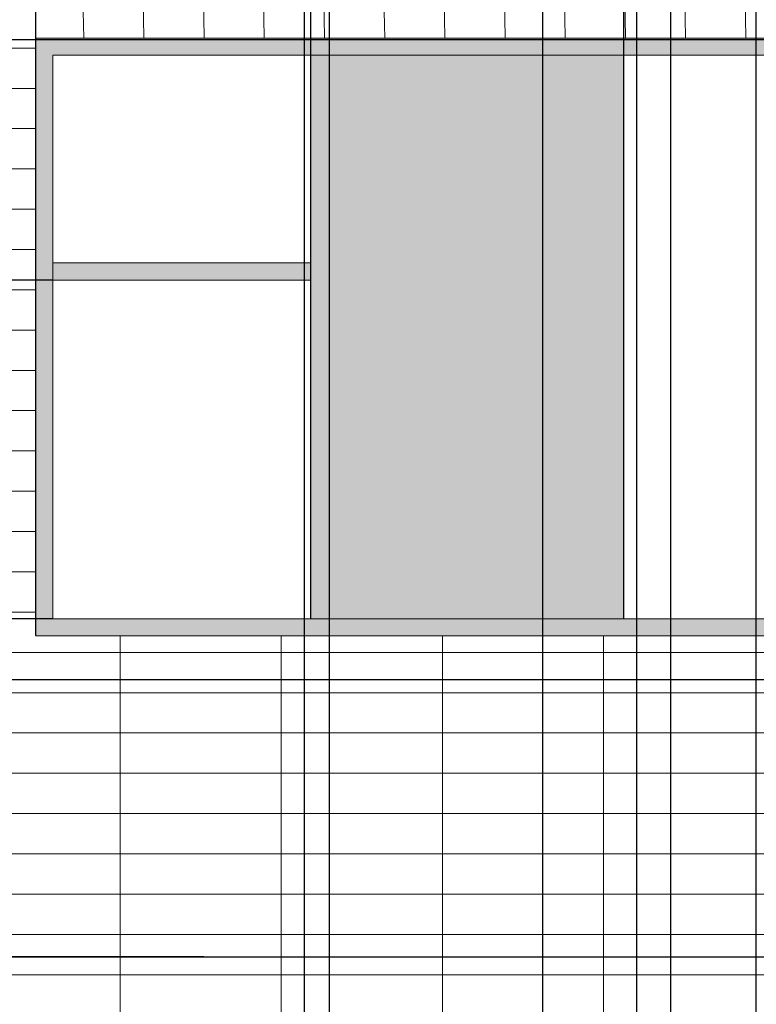
# Model space of a CAD drawing. Units: inches. Extents: x 241 to 943, y 109 to 1396.
# Tile 29 of 34: x 532 to 618, y 1065 to 1180. Entities that reach past the tile are written whole.
import ezdxf

# ---------------------------------------------------------------- set-up
doc = ezdxf.new("R2010")
doc.units = ezdxf.units.IN
doc.header["$MEASUREMENT"] = 0
for name, color, linetype, lineweight in [('A-ANNO-DIMS', 2, 'Continuous', 18), ('A-ELEV', 7, 'Continuous', 25), ('A-ELEV-SHAD', 9, 'Continuous', 13), ('A-GLAZ', 4, 'Continuous', 18), ('A-GLAZ-PATT', 18, 'Continuous', 13), ('A-WALL-PATT', 8, 'Continuous', 13)]:
    doc.layers.add(name, color=color, linetype=linetype, lineweight=lineweight)
doc.styles.get("Standard").update_dxf_attribs({"font": 'arial.ttf'})
doc.dimstyles.get("Standard").update_dxf_attribs({"dimtxt": 1.4375, "dimasz": 0.18, "dimexe": 0.18, "dimexo": 0.0625, "dimgap": 0.09, "dimtad": 0, "dimtih": 1, "dimtoh": 1, "dimdec": 4, "dimzin": 0, "dimdsep": 46, "dimlunit": 4, "dimtxsty": 'Standard', "dimcen": 0.09, "dimadec": 0, "dimazin": 0, "dimtfac": 1, "dimtdec": 4, "dimtofl": 0, "dimtmove": 0, "dimatfit": 3, "dimfxl": 1, "dimtolj": 1, "dimtzin": 0, "dimarcsym": 0})

# ---------------------------------------------------------------- blocks, each defined once
blk = doc.blocks.new('*D12')
at = {"layer": 'A-ANNO-DIMS', "color": 0, "lineweight": -2, "transparency": 16777216}
for p, q in [((530.23, 384.24), (530.23, 1395.05)), ((530.41, 1394.87), (587.56, 1394.87)), ((650.73, 1394.87), (593.58, 1394.87)), ((650.91, 384.24), (650.91, 1395.05))]:
    blk.add_line(p, q, dxfattribs=at)
at = {"layer": 'A-ANNO-DIMS', "color": 0, "transparency": 16777216}
for points in [[(530.41, 1394.9), (530.41, 1394.84), (530.23, 1394.87)], [(650.73, 1394.9), (650.73, 1394.84), (650.91, 1394.87)]]:
    blk.add_solid(points, dxfattribs=at)
at = {"layer": 'Defpoints', "color": 0, "transparency": 16777216}
for p in [(650.91, 1394.87), (530.23, 384.18), (650.91, 384.18)]:
    blk.add_point(p, dxfattribs=at)
at = {"layer": 'A-ANNO-DIMS', "color": 0, "transparency": 16777216, "insert": (590.57, 1394.87), "char_height": 1.438, "attachment_point": 5}
blk.add_mtext('\\A1;120.68', dxfattribs=at)
blk = doc.blocks.new('*D49')
at = {"layer": 'A-ANNO-DIMS', "color": 0, "lineweight": -2, "transparency": 16777216}
for p, q in [((766.24, 1177.54), (244.31, 1177.54)), ((244.49, 1177.36), (244.49, 1141.12)), ((244.49, 1103.23), (244.49, 1139.47)), ((766.24, 1103.05), (244.31, 1103.05))]:
    blk.add_line(p, q, dxfattribs=at)
at = {"layer": 'A-ANNO-DIMS', "color": 0, "transparency": 16777216}
for points in [[(244.46, 1177.36), (244.52, 1177.36), (244.49, 1177.54)], [(244.46, 1103.23), (244.52, 1103.23), (244.49, 1103.05)]]:
    blk.add_solid(points, dxfattribs=at)
at = {"layer": 'Defpoints', "color": 0, "transparency": 16777216}
for p in [(244.49, 1177.54), (766.3, 1177.54), (766.3, 1103.05)]:
    blk.add_point(p, dxfattribs=at)
at = {"layer": 'A-ANNO-DIMS', "color": 0, "transparency": 16777216, "insert": (244.49, 1140.29), "char_height": 1.438, "attachment_point": 5}
blk.add_mtext('\\A1;74.49', dxfattribs=at)
blk = doc.blocks.new('*D57')
at = {"layer": 'A-ANNO-DIMS', "color": 0, "lineweight": -2, "transparency": 16777216}
for p, q in [((508.31, 1070.92), (508.31, 1395.05)), ((508.49, 1394.87), (518.04, 1394.87)), ((533.77, 1394.87), (524.21, 1394.87)), ((533.95, 1108.23), (533.95, 1395.05))]:
    blk.add_line(p, q, dxfattribs=at)
at = {"layer": 'A-ANNO-DIMS', "color": 0, "transparency": 16777216}
for points in [[(508.49, 1394.9), (508.49, 1394.84), (508.31, 1394.87)], [(533.77, 1394.9), (533.77, 1394.84), (533.95, 1394.87)]]:
    blk.add_solid(points, dxfattribs=at)
at = {"layer": 'Defpoints', "color": 0, "transparency": 16777216}
for p in [(533.95, 1394.87), (533.95, 1108.17), (508.31, 1070.85)]:
    blk.add_point(p, dxfattribs=at)
at = {"layer": 'A-ANNO-DIMS', "color": 0, "transparency": 16777216, "insert": (521.13, 1394.87), "char_height": 1.438, "attachment_point": 5}
blk.add_mtext('\\A1;25.646', dxfattribs=at)
blk = doc.blocks.new('*D62')
at = {"layer": 'A-ANNO-DIMS', "color": 0, "lineweight": -2, "transparency": 16777216}
for p, q in [((424.11, 568.89), (424.11, 1395.05)), ((424.29, 1394.87), (492.35, 1394.87)), ((565.02, 1394.87), (496.96, 1394.87)), ((565.2, 568.89), (565.2, 1395.05))]:
    blk.add_line(p, q, dxfattribs=at)
at = {"layer": 'A-ANNO-DIMS', "color": 0, "transparency": 16777216}
for points in [[(424.29, 1394.9), (424.29, 1394.84), (424.11, 1394.87)], [(565.02, 1394.9), (565.02, 1394.84), (565.2, 1394.87)]]:
    blk.add_solid(points, dxfattribs=at)
at = {"layer": 'Defpoints', "color": 0, "transparency": 16777216}
for p in [(565.2, 1394.87), (424.11, 568.83), (565.2, 568.83)]:
    blk.add_point(p, dxfattribs=at)
at = {"layer": 'A-ANNO-DIMS', "color": 0, "transparency": 16777216, "insert": (494.66, 1394.87), "char_height": 1.438, "attachment_point": 5}
blk.add_mtext('\\A1;141.1', dxfattribs=at)
blk = doc.blocks.new('*D65')
at = {"layer": 'A-ANNO-DIMS', "color": 0, "lineweight": -2, "transparency": 16777216}
for p, q in [((424.11, 700.85), (424.11, 1395.05)), ((424.29, 1394.87), (505.52, 1394.87)), ((592.77, 1394.87), (511.54, 1394.87)), ((592.95, 700.85), (592.95, 1395.05))]:
    blk.add_line(p, q, dxfattribs=at)
at = {"layer": 'A-ANNO-DIMS', "color": 0, "transparency": 16777216}
for points in [[(424.29, 1394.9), (424.29, 1394.84), (424.11, 1394.87)], [(592.77, 1394.9), (592.77, 1394.84), (592.95, 1394.87)]]:
    blk.add_solid(points, dxfattribs=at)
at = {"layer": 'Defpoints', "color": 0, "transparency": 16777216}
for p in [(592.95, 1394.87), (424.11, 700.79), (592.95, 700.79)]:
    blk.add_point(p, dxfattribs=at)
at = {"layer": 'A-ANNO-DIMS', "color": 0, "transparency": 16777216, "insert": (508.53, 1394.87), "char_height": 1.438, "attachment_point": 5}
blk.add_mtext('\\A1;168.85', dxfattribs=at)
blk = doc.blocks.new('*D66')
at = {"layer": 'A-ANNO-DIMS', "color": 0, "lineweight": -2, "transparency": 16777216}
for p, q in [((617.76, 702.85), (617.76, 1395.05)), ((617.94, 1394.87), (680.69, 1394.87)), ((749.45, 1394.87), (686.7, 1394.87)), ((749.63, 702.85), (749.63, 1395.05))]:
    blk.add_line(p, q, dxfattribs=at)
at = {"layer": 'A-ANNO-DIMS', "color": 0, "transparency": 16777216}
for points in [[(617.94, 1394.9), (617.94, 1394.84), (617.76, 1394.87)], [(749.45, 1394.9), (749.45, 1394.84), (749.63, 1394.87)]]:
    blk.add_solid(points, dxfattribs=at)
at = {"layer": 'Defpoints', "color": 0, "transparency": 16777216}
for p in [(749.63, 1394.87), (617.76, 702.79), (749.63, 702.79)]:
    blk.add_point(p, dxfattribs=at)
at = {"layer": 'A-ANNO-DIMS', "color": 0, "transparency": 16777216, "insert": (683.7, 1394.87), "char_height": 1.438, "attachment_point": 5}
blk.add_mtext('\\A1;131.87', dxfattribs=at)
blk = doc.blocks.new('*D67')
at = {"layer": 'A-ANNO-DIMS', "color": 0, "lineweight": -2, "transparency": 16777216}
for p, q in [((389.04, 773.55), (389.04, 1395.05)), ((389.22, 1394.87), (495.34, 1394.87)), ((607.64, 1394.87), (501.52, 1394.87)), ((607.82, 773.55), (607.82, 1395.05))]:
    blk.add_line(p, q, dxfattribs=at)
at = {"layer": 'A-ANNO-DIMS', "color": 0, "transparency": 16777216}
for points in [[(389.22, 1394.9), (389.22, 1394.84), (389.04, 1394.87)], [(607.64, 1394.9), (607.64, 1394.84), (607.82, 1394.87)]]:
    blk.add_solid(points, dxfattribs=at)
at = {"layer": 'Defpoints', "color": 0, "transparency": 16777216}
for p in [(607.82, 1394.87), (389.04, 773.49), (607.82, 773.49)]:
    blk.add_point(p, dxfattribs=at)
at = {"layer": 'A-ANNO-DIMS', "color": 0, "transparency": 16777216, "insert": (498.43, 1394.87), "char_height": 1.438, "attachment_point": 5}
blk.add_mtext('\\A1;218.77', dxfattribs=at)
blk = doc.blocks.new('*D68')
at = {"layer": 'A-ANNO-DIMS', "color": 0, "lineweight": -2, "transparency": 16777216}
for p, q in [((617.76, 841.6), (617.76, 1395.05)), ((617.94, 1394.87), (702.22, 1394.87)), ((792.51, 1394.87), (708.23, 1394.87)), ((792.69, 841.6), (792.69, 1395.05))]:
    blk.add_line(p, q, dxfattribs=at)
at = {"layer": 'A-ANNO-DIMS', "color": 0, "transparency": 16777216}
for points in [[(617.94, 1394.9), (617.94, 1394.84), (617.76, 1394.87)], [(792.51, 1394.9), (792.51, 1394.84), (792.69, 1394.87)]]:
    blk.add_solid(points, dxfattribs=at)
at = {"layer": 'Defpoints', "color": 0, "transparency": 16777216}
for p in [(792.69, 1394.87), (617.76, 841.54), (792.69, 841.54)]:
    blk.add_point(p, dxfattribs=at)
at = {"layer": 'A-ANNO-DIMS', "color": 0, "transparency": 16777216, "insert": (705.23, 1394.87), "char_height": 1.438, "attachment_point": 5}
blk.add_mtext('\\A1;174.93', dxfattribs=at)
blk = doc.blocks.new('*D69')
at = {"layer": 'A-ANNO-DIMS', "color": 0, "lineweight": -2, "transparency": 16777216}
for p, q in [((389.04, 941.55), (389.04, 1395.05)), ((389.22, 1394.87), (476.28, 1394.87)), ((567.95, 1394.87), (480.9, 1394.87)), ((568.13, 941.55), (568.13, 1395.05))]:
    blk.add_line(p, q, dxfattribs=at)
at = {"layer": 'A-ANNO-DIMS', "color": 0, "transparency": 16777216}
for points in [[(389.22, 1394.9), (389.22, 1394.84), (389.04, 1394.87)], [(567.95, 1394.9), (567.95, 1394.84), (568.13, 1394.87)]]:
    blk.add_solid(points, dxfattribs=at)
at = {"layer": 'Defpoints', "color": 0, "transparency": 16777216}
for p in [(568.13, 1394.87), (389.04, 941.49), (568.13, 941.49)]:
    blk.add_point(p, dxfattribs=at)
at = {"layer": 'A-ANNO-DIMS', "color": 0, "transparency": 16777216, "insert": (478.59, 1394.87), "char_height": 1.438, "attachment_point": 5}
blk.add_mtext('\\A1;179.1', dxfattribs=at)
blk = doc.blocks.new('*D70')
at = {"layer": 'A-ANNO-DIMS', "color": 0, "lineweight": -2, "transparency": 16777216}
for p, q in [((603.87, 1009.6), (603.87, 1395.05)), ((604.05, 1394.87), (674.69, 1394.87)), ((751.33, 1394.87), (680.69, 1394.87)), ((751.51, 1009.6), (751.51, 1395.05))]:
    blk.add_line(p, q, dxfattribs=at)
at = {"layer": 'A-ANNO-DIMS', "color": 0, "transparency": 16777216}
for points in [[(604.05, 1394.9), (604.05, 1394.84), (603.87, 1394.87)], [(751.33, 1394.9), (751.33, 1394.84), (751.51, 1394.87)]]:
    blk.add_solid(points, dxfattribs=at)
at = {"layer": 'Defpoints', "color": 0, "transparency": 16777216}
for p in [(751.51, 1394.87), (603.87, 1009.54), (751.51, 1009.54)]:
    blk.add_point(p, dxfattribs=at)
at = {"layer": 'A-ANNO-DIMS', "color": 0, "transparency": 16777216, "insert": (677.69, 1394.87), "char_height": 1.438, "attachment_point": 5}
blk.add_mtext('\\A1;147.64', dxfattribs=at)
blk = doc.blocks.new('*D82')
at = {"layer": 'A-ANNO-DIMS', "color": 0, "lineweight": -2, "transparency": 16777216}
for p, q in [((565.2, 568.89), (565.2, 1395.05)), ((565.38, 1394.87), (605.89, 1394.87)), ((651.42, 1394.87), (610.91, 1394.87)), ((651.6, 568.89), (651.6, 1395.05))]:
    blk.add_line(p, q, dxfattribs=at)
at = {"layer": 'A-ANNO-DIMS', "color": 0, "transparency": 16777216}
for points in [[(565.38, 1394.9), (565.38, 1394.84), (565.2, 1394.87)], [(651.42, 1394.9), (651.42, 1394.84), (651.6, 1394.87)]]:
    blk.add_solid(points, dxfattribs=at)
at = {"layer": 'Defpoints', "color": 0, "transparency": 16777216}
for p in [(651.6, 1394.87), (565.2, 568.83), (651.6, 568.83)]:
    blk.add_point(p, dxfattribs=at)
at = {"layer": 'A-ANNO-DIMS', "color": 0, "transparency": 16777216, "insert": (608.4, 1394.87), "char_height": 1.438, "attachment_point": 5}
blk.add_mtext('\\A1;86.40', dxfattribs=at)
blk = doc.blocks.new('*D83')
at = {"layer": 'A-ANNO-DIMS', "color": 0, "lineweight": -2, "transparency": 16777216}
for p, q in [((592.95, 700.85), (592.95, 1395.05)), ((593.13, 1394.87), (602.27, 1394.87)), ((617.58, 1394.87), (608.45, 1394.87)), ((617.76, 702.85), (617.76, 1395.05))]:
    blk.add_line(p, q, dxfattribs=at)
at = {"layer": 'A-ANNO-DIMS', "color": 0, "transparency": 16777216}
for points in [[(593.13, 1394.9), (593.13, 1394.84), (592.95, 1394.87)], [(617.58, 1394.9), (617.58, 1394.84), (617.76, 1394.87)]]:
    blk.add_solid(points, dxfattribs=at)
at = {"layer": 'Defpoints', "color": 0, "transparency": 16777216}
for p in [(617.76, 1394.87), (617.76, 702.79), (592.95, 700.79)]:
    blk.add_point(p, dxfattribs=at)
at = {"layer": 'A-ANNO-DIMS', "color": 0, "transparency": 16777216, "insert": (605.36, 1394.87), "char_height": 1.438, "attachment_point": 5}
blk.add_mtext('\\A1;24.805', dxfattribs=at)
blk = doc.blocks.new('*D89')
at = {"layer": 'A-ANNO-DIMS', "color": 0, "lineweight": -2, "transparency": 16777216}
for p, q in [((377.04, 841.6), (377.04, 1395.05)), ((377.22, 1394.87), (494.32, 1394.87)), ((617.58, 1394.87), (500.48, 1394.87)), ((617.76, 841.6), (617.76, 1395.05))]:
    blk.add_line(p, q, dxfattribs=at)
at = {"layer": 'A-ANNO-DIMS', "color": 0, "transparency": 16777216}
for points in [[(377.22, 1394.9), (377.22, 1394.84), (377.04, 1394.87)], [(617.58, 1394.9), (617.58, 1394.84), (617.76, 1394.87)]]:
    blk.add_solid(points, dxfattribs=at)
at = {"layer": 'Defpoints', "color": 0, "transparency": 16777216}
for p in [(617.76, 1394.87), (377.04, 841.54), (617.76, 841.54)]:
    blk.add_point(p, dxfattribs=at)
at = {"layer": 'A-ANNO-DIMS', "color": 0, "transparency": 16777216, "insert": (497.4, 1394.87), "char_height": 1.438, "attachment_point": 5}
blk.add_mtext('\\A1;240.72', dxfattribs=at)
blk = doc.blocks.new('*D90')
at = {"layer": 'A-ANNO-DIMS', "color": 0, "lineweight": -2, "transparency": 16777216}
for p, q in [((568.13, 941.55), (568.13, 1395.05)), ((568.31, 1394.87), (582.92, 1394.87)), ((603.69, 1394.87), (589.08, 1394.87)), ((603.87, 902.92), (603.87, 1395.05))]:
    blk.add_line(p, q, dxfattribs=at)
at = {"layer": 'A-ANNO-DIMS', "color": 0, "transparency": 16777216}
for points in [[(568.31, 1394.9), (568.31, 1394.84), (568.13, 1394.87)], [(603.69, 1394.9), (603.69, 1394.84), (603.87, 1394.87)]]:
    blk.add_solid(points, dxfattribs=at)
at = {"layer": 'Defpoints', "color": 0, "transparency": 16777216}
for p in [(603.87, 1394.87), (568.13, 941.49), (603.87, 902.85)]:
    blk.add_point(p, dxfattribs=at)
at = {"layer": 'A-ANNO-DIMS', "color": 0, "transparency": 16777216, "insert": (586, 1394.87), "char_height": 1.438, "attachment_point": 5}
blk.add_mtext('\\A1;35.735', dxfattribs=at)
blk = doc.blocks.new('*D95')
at = {"layer": 'A-ANNO-DIMS', "color": 0, "lineweight": -2, "transparency": 16777216}
for p, q in [((724.88, 1108.17), (940.6, 1108.17)), ((940.42, 1107.99), (940.42, 1090.34)), ((940.42, 1071.03), (940.42, 1088.69)), ((508.37, 1070.85), (940.6, 1070.85))]:
    blk.add_line(p, q, dxfattribs=at)
at = {"layer": 'A-ANNO-DIMS', "color": 0, "transparency": 16777216}
for points in [[(940.39, 1107.99), (940.45, 1107.99), (940.42, 1108.17)], [(940.39, 1071.03), (940.45, 1071.03), (940.42, 1070.85)]]:
    blk.add_solid(points, dxfattribs=at)
at = {"layer": 'Defpoints', "color": 0, "transparency": 16777216}
for p in [(724.82, 1108.17), (940.42, 1108.17), (508.31, 1070.85)]:
    blk.add_point(p, dxfattribs=at)
at = {"layer": 'A-ANNO-DIMS', "color": 0, "transparency": 16777216, "insert": (940.42, 1089.51), "char_height": 1.438, "attachment_point": 5}
blk.add_mtext('\\A1;37.315', dxfattribs=at)
blk = doc.blocks.new('*D99')
at = {"layer": 'A-ANNO-DIMS', "color": 0, "lineweight": -2, "transparency": 16777216}
for p, q in [((417.09, 181.71), (417.09, 1395.05)), ((417.27, 1394.87), (539.16, 1394.87)), ((667.21, 1394.87), (545.33, 1394.87)), ((667.39, 214.58), (667.39, 1395.05))]:
    blk.add_line(p, q, dxfattribs=at)
at = {"layer": 'A-ANNO-DIMS', "color": 0, "transparency": 16777216}
for points in [[(417.27, 1394.9), (417.27, 1394.84), (417.09, 1394.87)], [(667.21, 1394.9), (667.21, 1394.84), (667.39, 1394.87)]]:
    blk.add_solid(points, dxfattribs=at)
at = {"layer": 'Defpoints', "color": 0, "transparency": 16777216}
for p in [(667.39, 1394.87), (667.39, 214.52), (417.09, 181.65)]:
    blk.add_point(p, dxfattribs=at)
at = {"layer": 'A-ANNO-DIMS', "color": 0, "transparency": 16777216, "insert": (542.24, 1394.87), "char_height": 1.438, "attachment_point": 5}
blk.add_mtext('\\A1;250.30', dxfattribs=at)
blk = doc.blocks.new('*D104')
at = {"layer": 'A-ANNO-DIMS', "color": 0, "lineweight": -2, "transparency": 16777216}
for p, q in [((533.95, 1108.23), (533.95, 1395.05)), ((534.13, 1394.87), (546.87, 1394.87)), ((565.77, 1394.87), (553.03, 1394.87)), ((565.95, 1110.23), (565.95, 1395.05))]:
    blk.add_line(p, q, dxfattribs=at)
at = {"layer": 'A-ANNO-DIMS', "color": 0, "transparency": 16777216}
for points in [[(534.13, 1394.9), (534.13, 1394.84), (533.95, 1394.87)], [(565.77, 1394.9), (565.77, 1394.84), (565.95, 1394.87)]]:
    blk.add_solid(points, dxfattribs=at)
at = {"layer": 'Defpoints', "color": 0, "transparency": 16777216}
for p in [(565.95, 1394.87), (565.95, 1110.17), (533.95, 1108.17)]:
    blk.add_point(p, dxfattribs=at)
at = {"layer": 'A-ANNO-DIMS', "color": 0, "transparency": 16777216, "insert": (549.95, 1394.87), "char_height": 1.438, "attachment_point": 5}
blk.add_mtext('\\A1;31.995', dxfattribs=at)
blk = doc.blocks.new('*D105')
at = {"layer": 'A-ANNO-DIMS', "color": 0, "lineweight": -2, "transparency": 16777216}
for p, q in [((565.95, 1110.23), (565.95, 1395.05)), ((566.13, 1394.87), (581.08, 1394.87)), ((602.18, 1394.87), (587.23, 1394.87)), ((602.36, 1110.23), (602.36, 1395.05))]:
    blk.add_line(p, q, dxfattribs=at)
at = {"layer": 'A-ANNO-DIMS', "color": 0, "transparency": 16777216}
for points in [[(566.13, 1394.9), (566.13, 1394.84), (565.95, 1394.87)], [(602.18, 1394.9), (602.18, 1394.84), (602.36, 1394.87)]]:
    blk.add_solid(points, dxfattribs=at)
at = {"layer": 'Defpoints', "color": 0, "transparency": 16777216}
for p in [(602.36, 1394.87), (565.95, 1110.17), (602.36, 1110.17)]:
    blk.add_point(p, dxfattribs=at)
at = {"layer": 'A-ANNO-DIMS', "color": 0, "transparency": 16777216, "insert": (584.15, 1394.87), "char_height": 1.438, "attachment_point": 5}
blk.add_mtext('\\A1;36.415', dxfattribs=at)
blk = doc.blocks.new('*D106')
at = {"layer": 'A-ANNO-DIMS', "color": 0, "lineweight": -2, "transparency": 16777216}
for p, q in [((602.36, 1110.23), (602.36, 1395.05)), ((602.54, 1394.87), (608.99, 1394.87)), ((620.34, 1394.87), (613.89, 1394.87)), ((620.52, 1110.23), (620.52, 1395.05))]:
    blk.add_line(p, q, dxfattribs=at)
at = {"layer": 'A-ANNO-DIMS', "color": 0, "transparency": 16777216}
for points in [[(602.54, 1394.9), (602.54, 1394.84), (602.36, 1394.87)], [(620.34, 1394.9), (620.34, 1394.84), (620.52, 1394.87)]]:
    blk.add_solid(points, dxfattribs=at)
at = {"layer": 'Defpoints', "color": 0, "transparency": 16777216}
for p in [(620.52, 1394.87), (602.36, 1110.17), (620.52, 1110.17)]:
    blk.add_point(p, dxfattribs=at)
at = {"layer": 'A-ANNO-DIMS', "color": 0, "transparency": 16777216, "insert": (611.44, 1394.87), "char_height": 1.438, "attachment_point": 5}
blk.add_mtext('\\A1;18.16', dxfattribs=at)
blk = doc.blocks.new('*D110')
at = {"layer": 'A-ANNO-DIMS', "color": 0, "lineweight": -2, "transparency": 16777216}
for p, q in [((535.89, 1149.58), (244.31, 1149.58)), ((244.49, 1149.4), (244.49, 1130.7)), ((244.49, 1110.35), (244.49, 1129.05)), ((535.89, 1110.17), (244.31, 1110.17))]:
    blk.add_line(p, q, dxfattribs=at)
at = {"layer": 'A-ANNO-DIMS', "color": 0, "transparency": 16777216}
for points in [[(244.46, 1149.4), (244.52, 1149.4), (244.49, 1149.58)], [(244.46, 1110.35), (244.52, 1110.35), (244.49, 1110.17)]]:
    blk.add_solid(points, dxfattribs=at)
at = {"layer": 'Defpoints', "color": 0, "transparency": 16777216}
for p in [(244.49, 1149.58), (535.95, 1149.58), (535.95, 1110.17)]:
    blk.add_point(p, dxfattribs=at)
at = {"layer": 'A-ANNO-DIMS', "color": 0, "transparency": 16777216, "insert": (244.49, 1129.87), "char_height": 1.438, "attachment_point": 5}
blk.add_mtext('\\A1;39.41', dxfattribs=at)
blk = doc.blocks.new('*D113')
at = {"layer": 'A-ANNO-DIMS', "color": 0, "lineweight": -2, "transparency": 16777216}
for p, q in [((603.87, 902.92), (603.87, 1395.05)), ((604.05, 1394.87), (618.91, 1394.87)), ((639.93, 1394.87), (625.07, 1394.87)), ((640.11, 902.92), (640.11, 1395.05))]:
    blk.add_line(p, q, dxfattribs=at)
at = {"layer": 'A-ANNO-DIMS', "color": 0, "transparency": 16777216}
for points in [[(604.05, 1394.9), (604.05, 1394.84), (603.87, 1394.87)], [(639.93, 1394.9), (639.93, 1394.84), (640.11, 1394.87)]]:
    blk.add_solid(points, dxfattribs=at)
at = {"layer": 'Defpoints', "color": 0, "transparency": 16777216}
for p in [(640.11, 1394.87), (603.87, 902.85), (640.11, 902.85)]:
    blk.add_point(p, dxfattribs=at)
at = {"layer": 'A-ANNO-DIMS', "color": 0, "transparency": 16777216, "insert": (621.99, 1394.87), "char_height": 1.438, "attachment_point": 5}
blk.add_mtext('\\A1;36.245', dxfattribs=at)

msp = doc.modelspace()

# ---------------------------------------------------------------- hatches: boundary and pattern name
at = {"layer": 'A-ELEV-SHAD'}
h = msp.add_hatch(color=256, dxfattribs=at)
h.dxf.hatch_style = 1
h.paths.add_polyline_path([(537.4269, 698.7912), (534.1778, 698.7912), (534.1778, 659.3434), (537.4269, 659.3434)])
h.paths.add_polyline_path([(508.0803, 698.7912), (450.9259, 698.7912), (450.9259, 659.3434), (452.9259, 659.3434), (452.9259, 696.7912), (506.0803, 696.7912), (506.0803, 659.3434), (508.0803, 659.3434)])
h.paths.add_polyline_path([(481.5031, 696.7912), (479.5031, 696.7912), (479.5031, 659.3434), (481.5031, 659.3434)], flags=17)
h.paths.add_polyline_path([(481.5031, 657.3434), (479.5031, 657.3434), (479.5031, 653.3371), (481.5031, 653.3371)], flags=17)
h.paths.add_polyline_path([(508.0803, 657.3434), (506.0803, 657.3434), (506.0803, 653.3371), (452.9259, 653.3371), (452.9259, 657.3434), (450.9259, 657.3434), (450.9259, 651.3371), (508.0803, 651.3371)])
h.paths.add_polyline_path([(428.1173, 839.5382), (426.1173, 839.5382), (426.1173, 786.9154), (428.1173, 786.9154)], flags=17)
h.paths.add_polyline_path([(470.8692, 839.5382), (468.8692, 839.5382), (468.8692, 786.9154), (470.8692, 786.9154)], flags=17)
h.paths.add_polyline_path([(508.3064, 841.5382), (396.3125, 841.5382), (396.3125, 782.5808), (398.3125, 782.5808), (398.3125, 839.5382), (506.3064, 839.5382), (506.3064, 782.5808), (508.3064, 782.5808)])
h.paths.add_polyline_path([(398.3125, 780.5808), (396.3125, 780.5808), (396.3125, 773.4916), (398.3125, 773.4916)])
h.paths.add_polyline_path([(508.3064, 780.5808), (506.3064, 780.5808), (506.3064, 773.4916), (508.3064, 773.4916)])
h.paths.add_polyline_path([(715.6236, 841.5382), (678.2674, 841.5382), (678.2674, 734.8538), (715.6236, 734.8538)])
h.paths.add_polyline_path([(680.2674, 839.5382), (682.4526, 839.5382), (713.6236, 839.5382), (713.6236, 736.9235), (690.2047, 736.9235), (680.2674, 736.9235)], flags=16)
h.paths.add_polyline_path([(792.691, 841.5382), (747.7579, 841.5382), (747.7579, 734.8538), (754.5373, 734.8538), (754.5373, 736.9235), (754.5373, 839.5382), (756.7224, 839.5382), (787.8934, 839.5382), (787.8934, 765.9585), (792.691, 765.9585)])
h.paths.add_polyline_path([(659.2925, 1009.5382), (657.2925, 1009.5382), (657.2925, 902.8538), (659.2925, 902.8538)])
h.paths.add_polyline_path([(751.5078, 976.6275), (712.5839, 976.6275), (712.5839, 974.6275), (751.5078, 974.6275)])
h.paths.add_polyline_path([(470.8692, 1007.5382), (468.8692, 1007.5382), (468.8692, 954.9154), (470.8692, 954.9154)], flags=17)
h.paths.add_polyline_path([(508.3064, 1009.5382), (396.3125, 1009.5382), (396.3125, 950.5808), (398.3125, 950.5808), (398.3125, 1007.5382), (506.3064, 1007.5382), (506.3064, 950.5808), (508.3064, 950.5808)])
h.paths.add_polyline_path([(428.1173, 1007.5382), (426.1173, 1007.5382), (426.1173, 954.9154), (428.1173, 954.9154)], flags=17)
h.paths.add_polyline_path([(398.3125, 948.5808), (396.3125, 948.5808), (396.3125, 941.4916), (398.3125, 941.4916)])
h.paths.add_polyline_path([(508.3064, 948.5808), (506.3064, 948.5808), (506.3064, 941.4916), (508.3064, 941.4916)])
h.paths.add_polyline_path([(428.1173, 1175.5382), (426.1173, 1175.5382), (426.1173, 1122.9154), (428.1173, 1122.9154)], flags=17)
h.paths.add_polyline_path([(508.3064, 1177.5382), (396.3125, 1177.5382), (396.3125, 1118.5808), (398.3125, 1118.5808), (398.3125, 1175.5382), (506.3064, 1175.5382), (506.3064, 1118.5808), (506.8039, 1118.5808, -1), (506.8039, 1116.5808), (506.3064, 1116.5808), (506.3064, 1109.4916), (508.3064, 1109.4916)])
h.paths.add_polyline_path([(470.8692, 1175.5382), (468.8692, 1175.5382), (468.8692, 1122.9154), (470.8692, 1122.9154)], flags=17)
h.paths.add_polyline_path([(398.3125, 1116.5808), (396.3125, 1116.5808), (396.3125, 1109.4916), (398.3125, 1109.4916)], flags=17)
h.paths.add_polyline_path([(724.819, 1177.7336), (533.952, 1177.7336), (533.952, 1108.1686), (724.819, 1108.1686)])
h.paths.add_polyline_path([(535.952, 1175.7336), (722.819, 1175.7336), (722.819, 1110.1686), (535.952, 1110.1686)], flags=0)
h.paths.add_polyline_path([(622.521, 1136.0739), (643.4534, 1136.0739), (643.4534, 1134.0739), (622.521, 1134.0739)], flags=0)
h.paths.add_polyline_path([(722.819, 1175.7336), (535.952, 1175.7336), (535.952, 1110.1686), (722.819, 1110.1686)], flags=16)
h.paths.add_polyline_path([(565.947, 1151.5772), (535.952, 1151.5772), (535.952, 1149.5772), (565.947, 1149.5772)], flags=0)
h = msp.add_hatch(color=256, dxfattribs=at)
h.dxf.hatch_style = 1
h.paths.add_polyline_path([(804.5268, 1142.2929), (768.3038, 1142.2929), (768.3038, 1140.2929), (804.5268, 1140.2929)], flags=0)
h.paths.add_polyline_path([(806.5268, 1177.5382), (766.3038, 1177.5382), (766.3038, 1103.0477), (806.5268, 1103.0477)])
h.paths.add_polyline_path([(768.3038, 1175.5382), (804.5268, 1175.5382), (804.5268, 1105.0477), (768.3038, 1105.0477)], flags=16)
h.paths.add_polyline_path([(643.4534, 1136.0739), (622.521, 1136.0739), (622.521, 1134.0739), (643.4534, 1134.0739)])
h.paths.add_polyline_path([(622.521, 1175.7336), (620.521, 1175.7336), (620.521, 1110.1686), (622.521, 1110.1686)])
h.paths.add_polyline_path([(565.947, 1151.5772), (535.952, 1151.5772), (535.952, 1149.5772), (565.947, 1149.5772)])
at = {"layer": 'A-GLAZ-PATT'}
h = msp.add_hatch(dxfattribs=at)
h.set_pattern_fill('GOST_GLASS', color=256, scale=0.89)
h.set_pattern_definition([(45, (0, 0), (7.5519, 0), [4.45, -6.23]), (45, (1.888, 0), (7.5519, 0), [1.78, -8.9]), (45, (0, 1.888), (7.5519, 0), [1.78, -8.9])])
h.paths.add_polyline_path([(676.8698, 700.7912), (652.0129, 700.7912), (652.0129, 628.4013), (676.8698, 628.4013)])
h.paths.add_polyline_path([(650.0129, 700.7912), (617.7594, 700.7912), (617.7594, 628.4013), (650.0129, 628.4013)])
h.paths.add_polyline_path([(747.7579, 841.5382), (715.6236, 841.5382), (715.6236, 734.8538), (747.7579, 734.8538)])
h.paths.add_polyline_path([(678.2674, 841.5382), (642.9197, 841.5382), (642.9197, 734.8538), (678.2674, 734.8538)])
h.paths.add_polyline_path([(712.5839, 1009.5382), (677.6886, 1009.5382), (677.6886, 902.8538), (712.5839, 902.8538)])
h.paths.add_polyline_path([(640.1141, 1009.5382), (603.8694, 1009.5382), (603.8694, 902.8538), (640.1141, 902.8538)])
h.paths.add_polyline_path([(682.8748, 1175.7336), (643.4534, 1175.7336), (643.4534, 1110.1686), (682.8748, 1110.1686)])
h.paths.add_polyline_path([(602.3616, 1175.7336), (565.947, 1175.7336), (565.947, 1110.1686), (602.3616, 1110.1686)])
h = msp.add_hatch(dxfattribs=at)
h.set_pattern_fill('ANSI31', color=256, scale=34, angle=45)
h.paths.add_polyline_path([(486.3418, 786.9154), (413.1187, 786.9154), (413.1187, 761.2284), (486.3418, 761.2284)])
h.paths.add_polyline_path([(486.3418, 954.9154), (413.1187, 954.9154), (413.1187, 929.2284), (486.3418, 929.2284)])
h.paths.add_polyline_path([(462.1074, 289.6933), (390.895, 289.6933), (390.895, 277.4626), (390.895, 274.3507), (462.1074, 274.3507), (462.1074, 277.4626)])
h.paths.add_polyline_path([(500.3323, 289.6933), (479.596, 289.6933), (479.596, 274.3507), (500.3323, 274.3507)])
h.paths.add_polyline_path([(450.9259, 566.8295), (426.1086, 566.8295), (426.1086, 498.4395), (446.4348, 498.4395), (446.4348, 519.3754), (450.9259, 519.3754), (450.9259, 525.3816), (445.5808, 525.3816, -1), (445.5808, 527.3816), (450.9259, 527.3816)])
h.paths.add_polyline_path([(563.2023, 508.9074), (534.1778, 508.9074), (508.1906, 508.9074), (508.1906, 498.4395), (563.2023, 498.4395)])
h.paths.add_polyline_path([(747.6328, 700.7912), (712.0171, 700.7912), (712.0171, 628.4013), (747.6328, 628.4013)])
h.paths.add_polyline_path([(446.4348, 643.7483), (426.1086, 643.7483), (426.1086, 630.4013), (446.4348, 630.4013)])
h.paths.add_polyline_path([(564.8076, 841.5382), (553.5166, 841.5382), (508.3064, 841.5382), (508.3064, 782.5808), (564.8076, 782.5808)])
h.paths.add_polyline_path([(564.8076, 780.5808), (508.3064, 780.5808), (508.3064, 773.4916), (564.8076, 773.4916)])
h.paths.add_polyline_path([(792.691, 762.5799), (759.6248, 762.5799), (759.6248, 736.9235), (759.6248, 734.8538), (792.691, 734.8538)])
h.paths.add_polyline_path([(564.8076, 1009.5382), (553.5166, 1009.5382), (508.3064, 1009.5382), (508.3064, 950.5808), (562.3033, 950.5808, -1), (562.3033, 948.5808), (508.3064, 948.5808), (508.3064, 941.4916), (564.8076, 941.4916)])
h.paths.add_polyline_path([(486.3418, 1122.9154), (413.1187, 1122.9154), (413.1187, 1097.2284), (486.3418, 1097.2284)])
at = {"layer": 'A-WALL-PATT'}
h = msp.add_hatch(dxfattribs=at)
h.set_pattern_fill('GRATE', color=256, scale=150)
h.paths.add_polyline_path([(747.7579, 1238.8538), (747.7579, 1275.9142), (747.7579, 1336.1154), (508.3064, 1336.1154), (508.3064, 1275.9142), (508.3064, 1238.8538), (508.3064, 1177.5382), (508.3064, 1109.4916), (508.3064, 1070.8538), (553.5166, 1070.8538), (749.6328, 1070.8538)])
h.paths.add_polyline_path([(533.952, 1108.1686), (533.952, 1177.7336), (533.952, 1303.0286), (724.819, 1303.0286), (724.819, 1108.1686)], flags=16)
h.paths.add_polyline_path([(535.952, 1110.1686), (535.952, 1175.7336), (722.819, 1175.7336), (722.819, 1110.1686)], flags=0)
h.paths.add_polyline_path([(643.4534, 1134.0739), (622.521, 1134.0739), (622.521, 1136.0739), (643.4534, 1136.0739)], flags=0)
h.paths.add_polyline_path([(617.7594, 568.8295), (617.7594, 734.8538), (377.0391, 734.8538), (377.0391, 566.8538), (377.0391, 400.8295), (417.0913, 400.8295), (618.9643, 400.8295)])
h.paths.add_polyline_path([(424.1086, 496.4395), (424.1086, 568.8295), (565.2023, 568.8295), (565.2023, 496.4395)], flags=16)
h.paths.add_polyline_path([(426.1086, 498.4395), (426.1086, 566.8295), (563.2023, 566.8295), (563.2023, 508.9074), (563.2023, 498.4395)], flags=0)
h.paths.add_polyline_path([(508.0803, 508.9074), (508.0803, 519.3754), (450.9259, 519.3754), (450.9259, 525.3816), (445.5808, 525.3816, -1), (445.5808, 527.3816), (450.9259, 527.3816), (450.9259, 566.8295), (508.0803, 566.8295), (537.4269, 566.8295), (537.4269, 508.9074)], flags=0)
h.paths.add_polyline_path([(506.0803, 521.3754), (452.9259, 521.3754), (452.9259, 564.8295), (506.0803, 564.8295)], flags=0)
h.paths.add_polyline_path([(424.1086, 628.4013), (424.1086, 700.7912), (592.9542, 700.7912), (592.9542, 628.4013)], flags=16)
h.paths.add_polyline_path([(426.1086, 630.4013), (426.1086, 698.7912), (590.8792, 698.7912), (590.8792, 630.4013)], flags=0)
h.paths.add_polyline_path([(508.1906, 651.3371), (508.0803, 651.3371), (450.9259, 651.3371), (428.0291, 651.3371), (428.0291, 698.7912), (451.9767, 698.7912), (508.0803, 698.7912), (537.4269, 698.7912), (563.2023, 698.7912), (563.2023, 659.3434), (563.9297, 659.3434), (563.9297, 651.3371)], flags=0)
h.paths.add_polyline_path([(506.0803, 653.3371), (452.9259, 653.3371), (452.9259, 657.3434), (445.5808, 657.3434, -1), (445.5808, 659.3434), (452.9259, 659.3434), (452.9259, 696.7912), (506.0803, 696.7912)], flags=0)
h = msp.add_hatch(dxfattribs=at)
h.set_pattern_fill('ANSI31', color=256, scale=56, angle=46)
h.paths.add_polyline_path([(508.3064, 1275.9142), (377.0391, 1275.9142), (377.0391, 1238.8538), (508.3064, 1238.8538)])
h.paths.add_polyline_path([(724.819, 1237.0695), (533.952, 1237.0695), (533.952, 1177.7336), (724.819, 1177.7336)])
h = msp.add_hatch(dxfattribs=at)
h.set_pattern_fill('GRATE', color=256, scale=150)
h.paths.add_polyline_path([(820.8374, 1070.8538), (749.6328, 1070.8538), (553.5166, 1070.8538), (508.3064, 1070.8538), (508.3064, 1009.5382), (553.5166, 1009.5382), (564.8076, 1009.5382), (603.8694, 1009.5382), (751.5078, 1009.5382), (751.5078, 902.8538), (603.8694, 902.8538), (603.8694, 1009.5382), (564.8076, 1009.5382), (564.8076, 941.4916), (568.1348, 941.4916), (568.1348, 902.8538), (581.3632, 902.8538), (581.3632, 841.5382), (564.8076, 841.5382), (564.8076, 782.5808), (605.9087, 782.5808, -1), (605.9087, 780.5808), (564.8076, 780.5808), (564.8076, 773.4916), (597.514, 773.4916), (607.8162, 773.4916), (607.8162, 734.8538), (617.7594, 734.8538), (617.7594, 841.5382), (792.691, 841.5382), (792.691, 734.8538), (617.7594, 734.8538), (617.7594, 702.7912), (749.6328, 702.7912), (749.6328, 626.4013), (617.7594, 626.4013), (617.7594, 568.8295), (820.8374, 568.8295), (820.8374, 736.8295), (820.8374, 902.8538)])

# ---------------------------------------------------------------- linework, layer by layer
at = {"layer": 'A-ELEV'}
for q in [(377.0391, 1070.8538), (749.6328, 1070.8538)]:
    msp.add_line((553.5166, 1070.8538), q, dxfattribs=at)
at = {"layer": 'A-GLAZ'}
for p, q in [((565.947, 1175.7336), (565.947, 1110.1686)), ((602.3616, 1175.7336), (602.3616, 1110.1686)), ((535.952, 1151.5772), (565.947, 1151.5772)), ((535.952, 1149.5772), (565.947, 1149.5772))]:
    msp.add_line(p, q, dxfattribs=at)
for points in [[(533.952, 1303.0286), (724.819, 1303.0286), (724.819, 1108.1686), (533.952, 1108.1686)], [(533.952, 1177.7336), (724.819, 1177.7336), (724.819, 1108.1686), (533.952, 1108.1686)], [(535.952, 1175.7336), (722.819, 1175.7336), (722.819, 1110.1686), (535.952, 1110.1686)]]:
    msp.add_lwpolyline(points, close=True, dxfattribs=at)

# ---------------------------------------------------------------- dimensions: what is measured, and where the dimension line sits
at = {"layer": 'A-ANNO-DIMS'}
for base, p1, p2, override, picture, middle in [((617.7594, 1394.8654), (377.0391, 841.5382), (617.7594, 841.5382), {"dimdec": 2, "dimlfac": 1, "dimrnd": 0, "dimzin": 0, "dimdsep": 46, "dimlunit": 2}, '*D89', (497.3993, 1394.8654)), ((607.8162, 1394.8654), (389.0429, 773.4916), (607.8162, 773.4916), {"dimdec": 2, "dimlfac": 1, "dimrnd": 0, "dimzin": 0, "dimdsep": 46, "dimlunit": 2}, '*D67', (498.4295, 1394.8654)), ((568.1348, 1394.8654), (389.0429, 941.4916), (568.1348, 941.4916), {"dimdec": 1, "dimlfac": 1, "dimrnd": 0, "dimzin": 0, "dimdsep": 46, "dimlunit": 2}, '*D69', (478.5888, 1394.8654)), ((667.3935, 1394.8654), (417.0913, 181.649), (667.3935, 214.5189), {"dimdec": 2, "dimlfac": 1, "dimrnd": 0, "dimzin": 0, "dimdsep": 46, "dimlunit": 2}, '*D99', (542.2424, 1394.8654)), ((565.2023, 1394.8654), (424.1086, 568.8295), (565.2023, 568.8295), {"dimdec": 1, "dimlfac": 1, "dimrnd": 0, "dimzin": 0, "dimdsep": 46, "dimlunit": 2}, '*D62', (494.6554, 1394.8654)), ((592.9542, 1394.8654), (424.1086, 700.7912), (592.9542, 700.7912), {"dimdec": 2, "dimlfac": 1, "dimrnd": 0, "dimzin": 0, "dimdsep": 46, "dimlunit": 2}, '*D65', (508.5314, 1394.8654)), ((533.952, 1394.8654), (508.3064, 1070.8538), (533.952, 1108.1686), {"dimdec": 3, "dimlfac": 1, "dimrnd": 0, "dimzin": 0, "dimdsep": 46, "dimlunit": 2}, '*D57', (521.1292, 1394.8654)), ((650.907, 1394.8654), (530.2303, 384.1784), (650.907, 384.1784), {"dimdec": 2, "dimlfac": 1, "dimrnd": 0, "dimzin": 0, "dimdsep": 46, "dimlunit": 2}, '*D12', (590.5686, 1394.8654)), ((565.947, 1394.8654), (533.952, 1108.1686), (565.947, 1110.1686), {"dimdec": 3, "dimlfac": 1, "dimrnd": 0, "dimzin": 0, "dimdsep": 46, "dimlunit": 2}, '*D104', (549.9495, 1394.8654)), ((651.5974, 1394.8654), (565.2023, 568.8295), (651.5974, 568.8295), {"dimdec": 2, "dimlfac": 1, "dimrnd": 0, "dimzin": 0, "dimdsep": 46, "dimlunit": 2}, '*D82', (608.3998, 1394.8654)), ((602.3616, 1394.8654), (565.947, 1110.1686), (602.3616, 1110.1686), {"dimdec": 3, "dimlfac": 1, "dimrnd": 0, "dimzin": 0, "dimdsep": 46, "dimlunit": 2}, '*D105', (584.1543, 1394.8654)), ((603.8694, 1394.8654), (568.1348, 941.4916), (603.8694, 902.8538), {"dimdec": 3, "dimlfac": 1, "dimrnd": 0, "dimzin": 0, "dimdsep": 46, "dimlunit": 2}, '*D90', (586.0021, 1394.8654)), ((617.7594, 1394.8654), (592.9542, 700.7912), (617.7594, 702.7912), {"dimdec": 3, "dimlfac": 1, "dimrnd": 0, "dimzin": 0, "dimdsep": 46, "dimlunit": 2}, '*D83', (605.3568, 1394.8654)), ((620.521, 1394.8654), (602.3616, 1110.1686), (620.521, 1110.1686), {"dimdec": 2, "dimlfac": 1, "dimrnd": 0, "dimzin": 0, "dimdsep": 46, "dimlunit": 2}, '*D106', (611.4413, 1394.8654)), ((751.5078, 1394.8654), (603.8694, 1009.5382), (751.5078, 1009.5382), {"dimdec": 2, "dimlfac": 1, "dimrnd": 0, "dimzin": 0, "dimdsep": 46, "dimlunit": 2}, '*D70', (677.6886, 1394.8654)), ((640.1141, 1394.8654), (603.8694, 902.8538), (640.1141, 902.8538), {"dimdec": 3, "dimlfac": 1, "dimrnd": 0, "dimzin": 0, "dimdsep": 46, "dimlunit": 2}, '*D113', (621.9918, 1394.8654)), ((749.6328, 1394.8654), (617.7594, 702.7912), (749.6328, 702.7912), {"dimdec": 2, "dimlfac": 1, "dimrnd": 0, "dimzin": 0, "dimdsep": 46, "dimlunit": 2}, '*D66', (683.6961, 1394.8654)), ((792.691, 1394.8654), (617.7594, 841.5382), (792.691, 841.5382), {"dimdec": 2, "dimlfac": 1, "dimrnd": 0, "dimzin": 0, "dimdsep": 46, "dimlunit": 2}, '*D68', (705.2252, 1394.8654))]:
    dim = msp.add_linear_dim(base=base, p1=p1, p2=p2, dimstyle='Standard', override=override, dxfattribs=at)
    dim.commit()
    dim.dimension.update_dxf_attribs({"geometry": picture, "text_midpoint": middle})
for base, p1, p2, override, picture, middle in [((244.4858, 1177.5382), (766.3038, 1103.0477), (766.3038, 1177.5382), {"dimdec": 2, "dimlfac": 1, "dimrnd": 0, "dimzin": 0, "dimdsep": 46, "dimlunit": 2}, '*D49', (244.4858, 1140.2929)), ((244.4858, 1149.5772), (535.952, 1110.1686), (535.952, 1149.5772), {"dimdec": 2, "dimlfac": 1, "dimrnd": 0, "dimzin": 0, "dimdsep": 46, "dimlunit": 2}, '*D110', (244.4858, 1129.8729)), ((940.417, 1108.1686), (508.3064, 1070.8538), (724.819, 1108.1686), {"dimdec": 3, "dimlfac": 1, "dimrnd": 0, "dimzin": 0, "dimdsep": 46, "dimlunit": 2}, '*D95', (940.417, 1089.5112))]:
    dim = msp.add_linear_dim(base=base, p1=p1, p2=p2, angle=90, dimstyle='Standard', override=override, dxfattribs=at)
    dim.commit()
    dim.dimension.update_dxf_attribs({"geometry": picture, "text_midpoint": middle})

doc.saveas('drawing.dxf')
